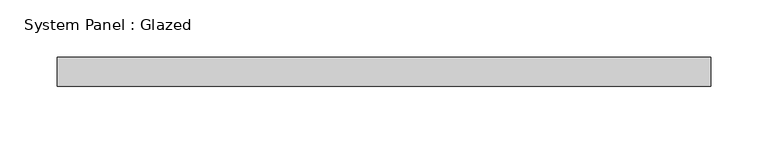
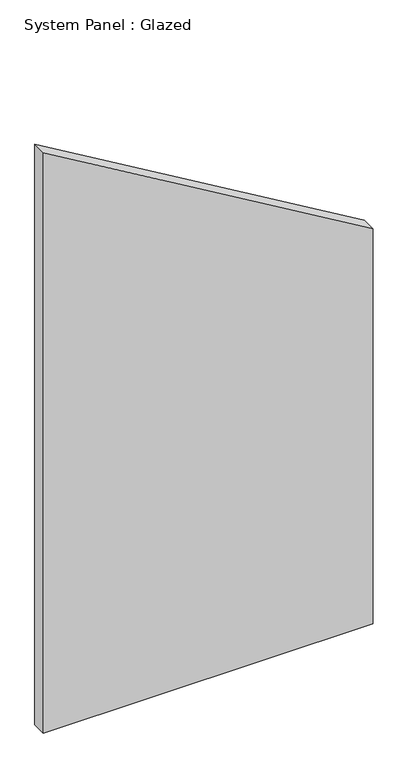
"""IFC4 building model written with IfcOpenShell, lengths in millimetres: plate geometry, System Panel : Glazed."""

from ifc_helpers import new_model, si_unit, frame, origin, place, context, project, spatial, polyline, outline, extrude, source, transform, mapped, element, save


def system_panel_glazed_cec062fa(model_context):
    return source(origin(), model_context, "Body", "SweptSolid", [
        extrude(outline(polyline([(0.0, -285.75), (0.0, 285.75), (722.9554653, 285.75), (1062.6231736, -285.75), (0.0, -285.75)])), frame((0.0, 19.05, 0.0), z_axis=(0.0, 1.0, 0.0), x_axis=(0.0, 0.0, 1.0)), (0.0, 0.0, 1.0), 25.4),
    ])


if __name__ == "__main__":
    model = new_model("IFC4")
    model_context = context("Model", 3, world=origin())
    ifc_project = project(units=[si_unit("LENGTHUNIT", "METRE", prefix="MILLI")], contexts=[model_context])
    site = spatial("IfcSite", under=ifc_project)
    building = spatial("IfcBuilding", under=site)
    placement = place(None, origin())
    system_panel_glazed_shape = system_panel_glazed_cec062fa(model_context)
    element("IfcPlate", 1, ObjectType="System Panel : Glazed", at=placement, inside=building, context=model_context, shape_type="MappedRepresentation", body=[
        mapped(system_panel_glazed_shape, transform((0.0, 0.0, 0.0), x_axis=(1.0, 0.0, 0.0), y_axis=(0.0, 1.0, 0.0), z_axis=(0.0, 0.0, 1.0))),
    ])
    save(model, "model.ifc")

# Revit data of these elements
# Type "System Panel : Glazed"
#   Construction Type Id = "GSP4R"
#   Analytic Construction = "1/8 in Pilkington single glazing"
#   Visual Light Transmittance = 0.9
#   Solar Heat Gain Coefficient = 0.86
#   Heat Transfer Coefficient (U) = 1.18115 BTU/(h·ft²·°F)
#   Define Thermal Properties by = 1
# Element 1 (IfcPlate, "System Panel : Glazed")
#   Materials on its faces: "Glass"
# Materials
#   "Glass": class "Glass", colour RGB 0 128 192, transparency 0.75, Description = "Soda Lime Glass", Cost = 0
